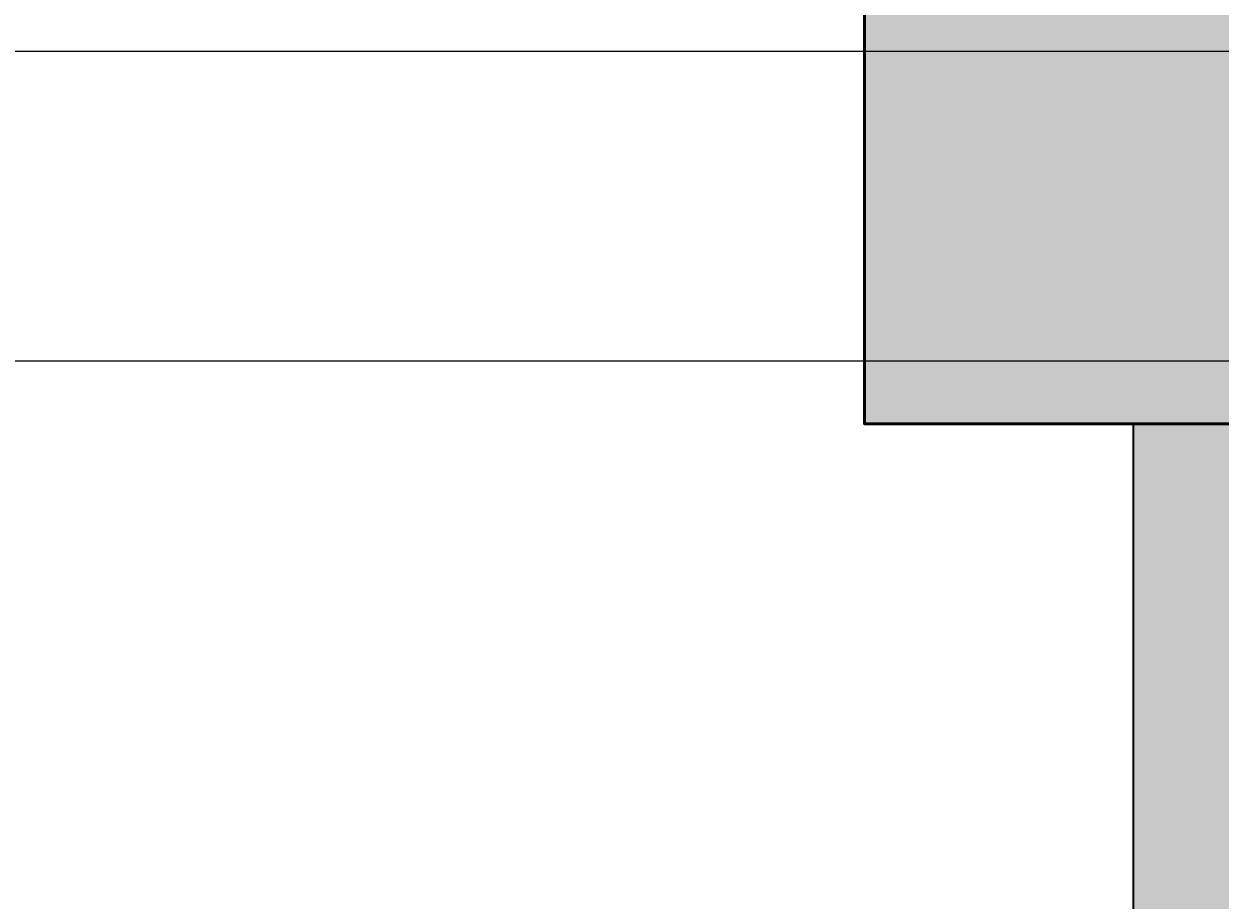
# Model space of a CAD drawing. Units: inches. Extents: x 1998 to 2588, y 1139 to 1977.
# Tile 51 of 134: x 2313 to 2344, y 1615 to 1637. Entities that reach past the tile are written whole.
import ezdxf

# ---------------------------------------------------------------- set-up
doc = ezdxf.new("R2010")
doc.units = ezdxf.units.IN
for name, color, linetype, lineweight in [('A-ANNO-DIMS', 2, 'Continuous', 18), ('A-COLS-PATT', 250, 'Continuous', 13), ('A-WALL-PATT', 252, 'Continuous', 13), ('COLUMN', 10, 'Continuous', 50), ('WALL', 200, 'Continuous', 35)]:
    doc.layers.add(name, color=color, linetype=linetype, lineweight=lineweight)
doc.styles.get("Standard").update_dxf_attribs({"font": 'arial.ttf'})
doc.dimstyles.get("Standard").update_dxf_attribs({"dimtxt": 0.18, "dimasz": 0.18, "dimexe": 0.18, "dimexo": 0.0625, "dimgap": 0.09, "dimtad": 0, "dimtih": 1, "dimtoh": 1, "dimdec": 4, "dimzin": 0, "dimdsep": 46, "dimtxsty": 'Standard', "dimcen": 0.09, "dimadec": 0, "dimazin": 0, "dimtfac": 1, "dimtdec": 4, "dimtofl": 0, "dimtmove": 0, "dimatfit": 3, "dimfxl": 1, "dimtolj": 1, "dimtzin": 0, "dimarcsym": 0})

# ---------------------------------------------------------------- blocks, each defined once
blk = doc.blocks.new('*D30')
at = {"layer": 'A-ANNO-DIMS', "color": 0, "lineweight": -2, "transparency": 16777216}
for p, q in [((2407.91, 1636.732), (1997.843, 1636.732)), ((1998.023, 1636.552), (1998.023, 1615.913)), ((1998.023, 1594.912), (1998.023, 1615.552)), ((2407.91, 1594.732), (1997.843, 1594.732))]:
    blk.add_line(p, q, dxfattribs=at)
at = {"layer": 'A-ANNO-DIMS', "color": 0, "transparency": 16777216}
for points in [[(1997.993, 1636.552), (1998.053, 1636.552), (1998.023, 1636.732)], [(1997.993, 1594.912), (1998.053, 1594.912), (1998.023, 1594.732)]]:
    blk.add_solid(points, dxfattribs=at)
at = {"layer": 'Defpoints', "color": 0, "transparency": 16777216}
for p in [(1998.023, 1636.732), (2407.973, 1636.732), (2407.973, 1594.732)]:
    blk.add_point(p, dxfattribs=at)
at = {"layer": 'A-ANNO-DIMS', "color": 0, "transparency": 16777216, "insert": (1998.023, 1615.732), "char_height": 0.18, "attachment_point": 5}
blk.add_mtext('\\A1;42', dxfattribs=at)
blk = doc.blocks.new('*D39')
at = {"layer": 'A-ANNO-DIMS', "color": 0, "lineweight": -2, "transparency": 16777216}
for p, q in [((2115.035, 1628.742), (2588.309, 1628.742)), ((2588.129, 1628.562), (2588.129, 1612.685)), ((2588.129, 1596.444), (2588.129, 1612.321)), ((2115.035, 1596.264), (2588.309, 1596.264))]:
    blk.add_line(p, q, dxfattribs=at)
at = {"layer": 'A-ANNO-DIMS', "color": 0, "transparency": 16777216}
for points in [[(2588.099, 1628.562), (2588.159, 1628.562), (2588.129, 1628.742)], [(2588.099, 1596.444), (2588.159, 1596.444), (2588.129, 1596.264)]]:
    blk.add_solid(points, dxfattribs=at)
at = {"layer": 'Defpoints', "color": 0, "transparency": 16777216}
for p in [(2114.973, 1628.742), (2588.129, 1628.742), (2114.973, 1596.264)]:
    blk.add_point(p, dxfattribs=at)
at = {"layer": 'A-ANNO-DIMS', "color": 0, "transparency": 16777216, "insert": (2588.129, 1612.503), "char_height": 0.18, "attachment_point": 5}
blk.add_mtext('\\A1;32.48', dxfattribs=at)

msp = doc.modelspace()

# ---------------------------------------------------------------- hatches: boundary and pattern name
at = {"layer": 'A-COLS-PATT'}
h = msp.add_hatch(color=256, dxfattribs=at)
h.dxf.hatch_style = 1
h.paths.add_polyline_path([(2099.4125, 1888.7324), (2087.9729, 1888.7324), (2087.9729, 1868.3278), (2099.4125, 1868.3278)])
h.paths.add_polyline_path([(2234.4125, 1888.7324), (2222.9729, 1888.7324), (2222.9729, 1868.3278), (2234.4125, 1868.3278)])
h.paths.add_polyline_path([(2341.4729, 1886.637), (2330.0332, 1886.637), (2330.0332, 1866.2324), (2341.4729, 1866.2324)])
h.paths.add_polyline_path([(2507.8006, 1882.7324), (2487.396, 1882.7324), (2487.396, 1871.2927), (2507.8006, 1871.2927)])
h.paths.add_polyline_path([(2510.9729, 1766.672), (2490.5682, 1766.672), (2490.5682, 1755.2324), (2510.9729, 1755.2324)])
h.paths.add_polyline_path([(2345.9729, 1759.7324), (2334.5332, 1759.7324), (2334.5332, 1739.3278), (2345.9729, 1739.3278)])
h.paths.add_polyline_path([(2234.4125, 1774.3318), (2222.9729, 1774.3318), (2222.9729, 1753.9272), (2234.4125, 1753.9272)])
h.paths.add_polyline_path([(2099.4125, 1775.637), (2087.9729, 1775.637), (2087.9729, 1755.2324), (2099.4125, 1755.2324)])
h.paths.add_polyline_path([(2098.0956, 1593.7241), (2077.691, 1593.7241), (2077.691, 1582.2845), (2098.0956, 1582.2845)])
h.paths.add_polyline_path([(2227.4729, 1604.637), (2216.0332, 1604.637), (2216.0332, 1584.2324), (2227.4729, 1584.2324)])
h.paths.add_polyline_path([(2345.9729, 1647.5211), (2334.5332, 1647.5211), (2334.5332, 1627.1165), (2345.9729, 1627.1165)])
h.paths.add_polyline_path([(2522.3775, 1641.2324), (2501.9729, 1641.2324), (2501.9729, 1629.7927), (2522.3775, 1629.7927)])
h.paths.add_polyline_path([(2522.3775, 1480.7324), (2501.9729, 1480.7324), (2501.9729, 1469.2927), (2522.3775, 1469.2927)])
h.paths.add_polyline_path([(2345.9729, 1488.5616), (2334.5332, 1488.5616), (2334.5332, 1468.1569), (2345.9729, 1468.1569)])
h.paths.add_polyline_path([(2234.4125, 1486.137), (2227.4729, 1486.137), (2227.4729, 1465.7324), (2234.4125, 1465.7324)])
h.paths.add_polyline_path([(2227.4729, 1486.137), (2222.9729, 1486.137), (2222.9729, 1465.7324), (2227.4729, 1465.7324)])
h.paths.add_polyline_path([(2108.3775, 1470.2324), (2087.9729, 1470.2324), (2087.9729, 1458.7927), (2108.3775, 1458.7927)])
h.paths.add_polyline_path([(2096.9729, 1365.5012), (2087.9729, 1365.5012), (2087.9729, 1345.0966), (2096.9729, 1345.0966)])
h.paths.add_polyline_path([(2087.9729, 1365.5012), (2085.5332, 1365.5012), (2085.5332, 1345.0966), (2087.9729, 1345.0966)])
h.paths.add_polyline_path([(2234.4125, 1285.137), (2222.9729, 1285.137), (2222.9729, 1264.7324), (2234.4125, 1264.7324)])
h.paths.add_polyline_path([(2345.9729, 1285.137), (2334.5332, 1285.137), (2334.5332, 1264.7324), (2345.9729, 1264.7324)])
h.paths.add_polyline_path([(2503.1458, 1240.172), (2482.7412, 1240.172), (2482.7412, 1228.7324), (2503.1458, 1228.7324)])
h.paths.add_polyline_path([(2510.9729, 1369.172), (2490.5682, 1369.172), (2490.5682, 1357.7324), (2510.9729, 1357.7324)])
at = {"layer": 'A-WALL-PATT'}
h = msp.add_hatch(color=256, dxfattribs=at)
h.dxf.hatch_style = 1
h.paths.add_polyline_path([(2222.9729, 1888.7324), (2099.4125, 1888.7324), (2099.4125, 1879.7324), (2222.9729, 1879.7324)])
h.paths.add_polyline_path([(2096.9729, 1868.3278), (2087.9729, 1868.3278), (2087.9729, 1775.637), (2096.9729, 1775.637)])
h.paths.add_polyline_path([(2227.4729, 1868.3278), (2222.9729, 1868.3278), (2222.9729, 1774.3318), (2227.4729, 1774.3318)])
h.paths.add_polyline_path([(2188.3019, 1759.7324), (2138.6074, 1759.7324), (2099.4125, 1759.7324), (2099.4125, 1755.2324), (2176.9729, 1755.2324), (2188.3019, 1755.2324)])
h.paths.add_polyline_path([(2087.9729, 1759.7324), (2059.4729, 1759.7324), (2059.4729, 1702.7324), (2087.9729, 1702.7324), (2087.9729, 1707.2324), (2063.9729, 1707.2324), (2063.9729, 1755.2324), (2087.9729, 1755.2324)])
h.paths.add_polyline_path([(2096.9729, 1755.2324), (2087.9729, 1755.2324), (2087.9729, 1707.2324), (2096.9729, 1707.2324)])
h.paths.add_polyline_path([(2187.0461, 1707.2324), (2105.9729, 1707.2324), (2096.9729, 1707.2324), (2087.9729, 1707.2324), (2087.9729, 1702.7324), (2105.9729, 1702.7324), (2114.9729, 1702.7324), (2187.0461, 1702.7324)])
h.paths.add_polyline_path([(2181.4729, 1719.2028), (2176.9729, 1719.2028), (2176.9729, 1707.2324), (2181.4729, 1707.2324)])
h.paths.add_polyline_path([(2216.0332, 1588.7324), (2114.9729, 1588.7324), (2105.9729, 1588.7324), (2105.9729, 1584.2324), (2216.0332, 1584.2324)])
h.paths.add_polyline_path([(2077.691, 1588.7324), (2061.4729, 1588.7324), (2061.4729, 1584.2324), (2077.691, 1584.2324)])
h.paths.add_polyline_path([(2105.9729, 1588.7324), (2098.0956, 1588.7324), (2098.0956, 1584.2324), (2105.9729, 1584.2324)])
h.paths.add_polyline_path([(2114.9729, 1596.2642), (2110.1012, 1596.2642), (2105.9729, 1596.2642), (2105.9729, 1588.7324), (2114.9729, 1588.7324)])
h.paths.add_polyline_path([(2114.9729, 1584.2324), (2105.9729, 1584.2324), (2105.9729, 1580.249), (2110.1012, 1580.249), (2114.9729, 1580.249)])
h.paths.add_polyline_path([(2114.9729, 1547.7716), (2110.1012, 1547.7716, -0.0318759), (2105.9729, 1548.035), (2105.9729, 1470.2324), (2108.3775, 1470.2324), (2108.3775, 1465.7324), (2186.2943, 1465.7324), (2186.2943, 1470.2324), (2114.9729, 1470.2324)])
h.paths.add_polyline_path([(2227.4729, 1584.2324), (2222.9729, 1584.2324), (2222.9729, 1486.137), (2227.4729, 1486.137)])
h.paths.add_polyline_path([(2295.4138, 1593.2324), (2227.4729, 1593.2324), (2227.4729, 1588.7324), (2295.4138, 1588.7324), (2295.4138, 1591.8729)])
h.paths.add_polyline_path([(2345.9729, 1627.1165), (2341.4729, 1627.1165), (2341.4729, 1593.2324), (2337.2869, 1593.2324), (2337.2869, 1591.8729), (2337.2869, 1588.7324), (2345.9729, 1588.7324)])
h.paths.add_polyline_path([(2291.9729, 1588.7324), (2287.4729, 1588.7324), (2287.4729, 1522.7324), (2291.9729, 1522.7324)])
h.paths.add_polyline_path([(2291.9729, 1522.7324), (2287.4729, 1522.7324), (2227.4729, 1522.7324), (2227.4729, 1518.2324), (2291.9729, 1518.2324)])
h.paths.add_polyline_path([(2295.7347, 1519.5919), (2295.7347, 1522.7324), (2291.9729, 1522.7324), (2291.9729, 1518.2324), (2295.7347, 1518.2324)])
h.paths.add_polyline_path([(2345.9729, 1522.7324), (2337.6078, 1522.7324), (2337.6078, 1519.5919), (2337.6078, 1518.2324), (2341.4729, 1518.2324), (2341.4729, 1488.5616), (2345.9729, 1488.5616)])
h.paths.add_polyline_path([(2345.9729, 1468.1569), (2341.4729, 1468.1569), (2341.4729, 1374.2324), (2227.4729, 1374.2324), (2227.4729, 1369.7324), (2345.9729, 1369.7324)])
h.paths.add_polyline_path([(2345.9729, 1369.7324), (2341.4729, 1369.7324), (2341.4729, 1362.2324), (2345.9729, 1362.2324)])
h.paths.add_polyline_path([(2345.9729, 1317.7324), (2345.9729, 1322.2324), (2341.4729, 1322.2324), (2341.4729, 1285.137), (2345.9729, 1285.137)], flags=17)
h.paths.add_polyline_path([(2356.2096, 1322.2324), (2345.9729, 1322.2324), (2345.9729, 1317.7324), (2356.2096, 1317.7324), (2356.2096, 1319.3088)], flags=17)
h.paths.add_polyline_path([(2393.9729, 1322.2324), (2375.6999, 1322.2324), (2375.6999, 1319.3088, -0.0202458), (2375.636, 1317.7324), (2393.9729, 1317.7324)], flags=17)
h.paths.add_polyline_path([(2398.4729, 1322.2324), (2393.9729, 1322.2324), (2393.9729, 1317.7324), (2393.9729, 1237.7324), (2345.9729, 1237.7324), (2345.9729, 1264.7324), (2341.4729, 1264.7324), (2341.4729, 1228.7324), (2393.9729, 1228.7324), (2482.7412, 1228.7324), (2482.7412, 1237.7324), (2398.4729, 1237.7324), (2398.4729, 1297.1029)])
h.paths.add_polyline_path([(2398.4729, 1362.2324), (2393.9729, 1362.2324), (2393.9729, 1357.7324), (2398.4729, 1357.7324)])
h.paths.add_polyline_path([(2345.9729, 1329.7549), (2341.4729, 1329.7549), (2341.4729, 1322.2324), (2345.9729, 1322.2324)])

# ---------------------------------------------------------------- linework, layer by layer
at = {"layer": 'COLUMN'}
msp.add_lwpolyline([(2334.5332, 1647.5211), (2345.9729, 1647.5211), (2345.9729, 1627.1165), (2334.5332, 1627.1165)], close=True, dxfattribs=at)
at = {"layer": 'WALL'}
msp.add_line((2341.4729, 1627.1165), (2341.4729, 1593.2324), dxfattribs=at)

# ---------------------------------------------------------------- dimensions: what is measured, and where the dimension line sits
at = {"layer": 'A-ANNO-DIMS'}
for base, p1, p2, override, picture, middle in [((1998.0229, 1636.7324), (2407.9729, 1594.7324), (2407.9729, 1636.7324), {"dimdec": 0, "dimlfac": 1, "dimrnd": 0, "dimzin": 0, "dimdsep": 46, "dimlunit": 2}, '*D30', (1998.0229, 1615.7324)), ((2588.1286, 1628.7416), (2114.9729, 1596.2642), (2114.9729, 1628.7416), {"dimdec": 2, "dimlfac": 1, "dimrnd": 0, "dimzin": 0, "dimdsep": 46, "dimlunit": 2}, '*D39', (2588.1286, 1612.5029))]:
    dim = msp.add_linear_dim(base=base, p1=p1, p2=p2, angle=90, dimstyle='Standard', override=override, dxfattribs=at)
    dim.commit()
    dim.dimension.update_dxf_attribs({"geometry": picture, "text_midpoint": middle})

doc.saveas('drawing.dxf')
